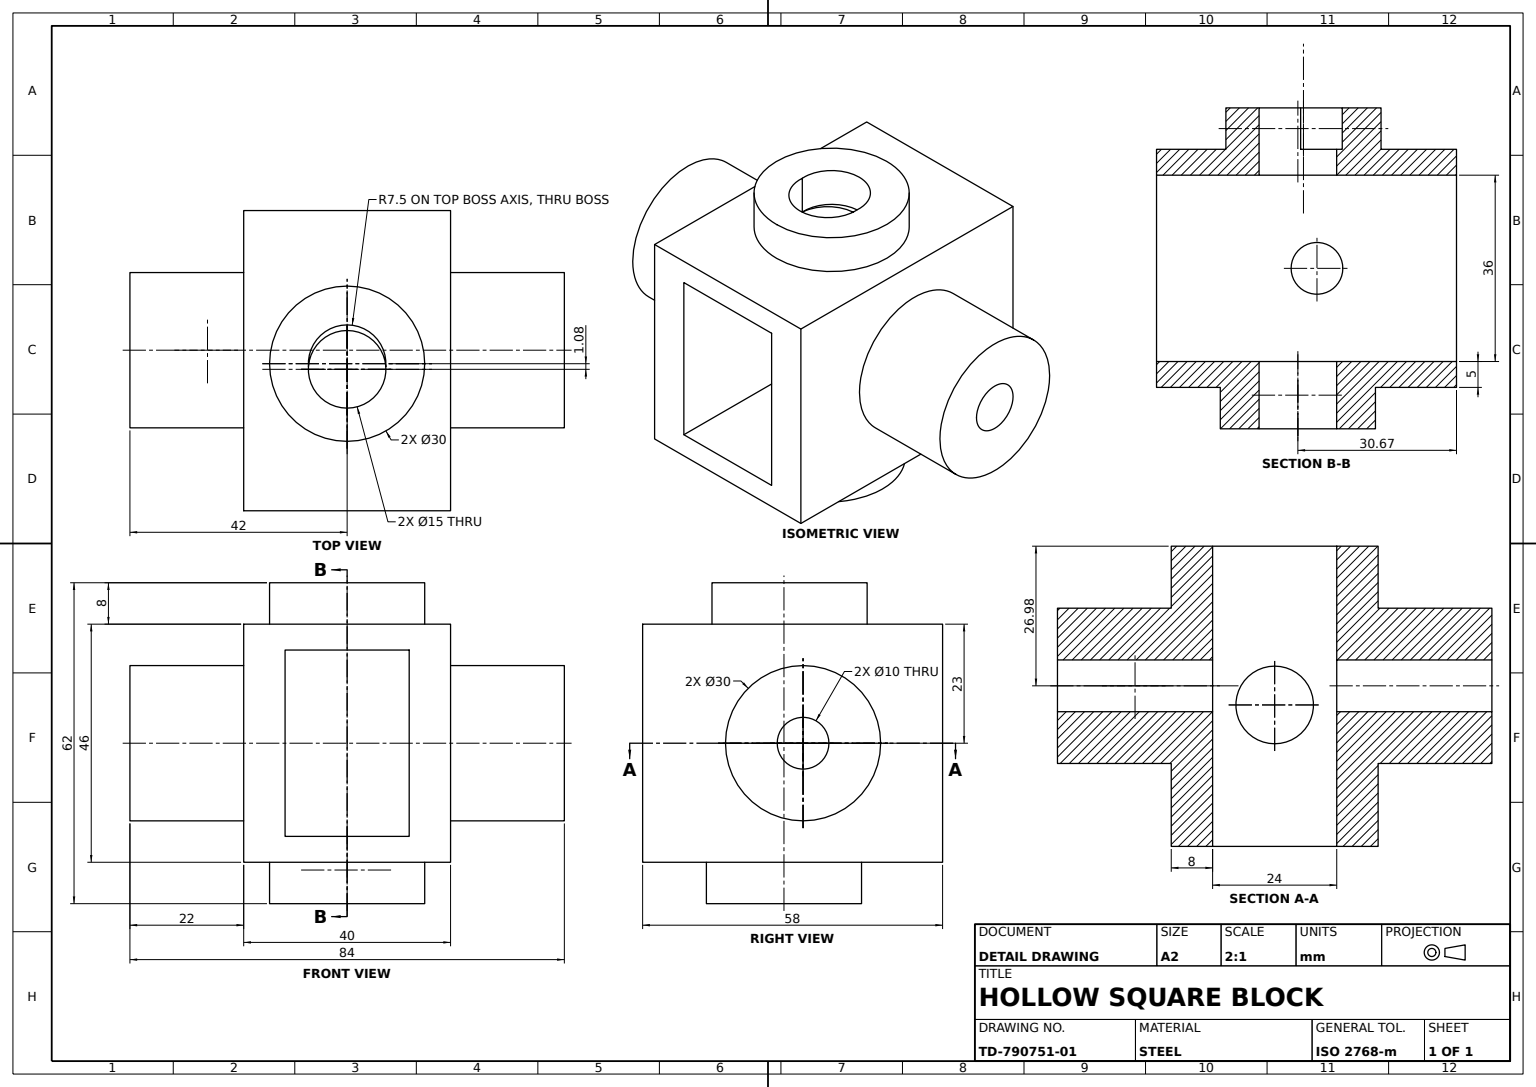
from build123d import *

# Parameters (mm, degrees)
VALVE_BODY_PROFILE_SKETCH_W  = 84
VALVE_BODY_PROFILE_SKETCH_H  = 46
VALVE_BODY_BLOCK_DEPTH       = 23
TOP_PORT_BOSS_SKETCH_R       = 15
TOP_PORT_BOSS_SKETCH_R_2     = 7.5
TOP_PORT_BOSS_30_DEPTH       = 8
BODY_WINDOW_SKETCH_W         = 24
BODY_WINDOW_SKETCH_H         = 36
BODY_WINDOW_CUT_24X36_DEPTH  = 60
SIDE_PORT_SKETCH_R           = 5
SIDE_PORT_THROUGH_BORE_DEPTH = 95
SKETCH4_3_R                  = 15
SKETCH4_3_R_2                = 5
SIDE_PORT_CUT_DEPTH          = 22
REAR_START                   = -22
REAR_PORT_SKETCH_W           = 46
REAR_PORT_SKETCH_H           = 46
REAR_PORT_SKETCH_R           = 15
REAR_PORT_CUT_DEPTH          = 22
FRONT_PORT_BOSS_SKETCH_R     = 15
FRONT_PORT_BOSS_SKETCH_R_2   = 7.5
FRONT_PORT_BOSS_30_DEPTH     = 8
FRONT_START                  = -61
SKETCH6_3_R                  = 7.5
FRONT_PORT_BORE_DEPTH        = 61


with BuildPart() as part:
    # Valve Body Profile Sketch → Valve Body Block (new, symmetric)
    with BuildSketch(Plane(origin=(0, 0, 0), x_dir=(1, 0, 0), z_dir=(0, 1, 0))):
        with Locations((0, 23)):
            Rectangle(VALVE_BODY_PROFILE_SKETCH_W, VALVE_BODY_PROFILE_SKETCH_H)
        Polygon((-20, 51.769982338), (20, 51.769982338), (20, 22.392939221), (20, -6.230017662), (-20, -6.230017662), (-20, 23), align=None)
    extrude(amount=VALVE_BODY_BLOCK_DEPTH, both=True)

    # Top Port Boss Sketch → Top Port Boss _30 (add)
    with BuildSketch(Plane(origin=(0, 23, 0), x_dir=(1, 0, 0), z_dir=(0, 1, 0))):
        with Locations(Location((0, 22.179634707, 0), (0, 0, 270))):
            Circle(TOP_PORT_BOSS_SKETCH_R)
        with Locations(Location((0, 22.179634707, 0), (0, 0, 270))):
            Circle(TOP_PORT_BOSS_SKETCH_R_2, mode=Mode.SUBTRACT)
    extrude(amount=TOP_PORT_BOSS_30_DEPTH)

    # Body Window Sketch → Body Window Cut 24x36 (cut)
    with BuildSketch(Plane.XY.offset(6.230017662)):
        Rectangle(BODY_WINDOW_SKETCH_W, BODY_WINDOW_SKETCH_H)
    extrude(amount=-BODY_WINDOW_CUT_24X36_DEPTH, mode=Mode.SUBTRACT)

    # Side Port Sketch → Side Port Through Bore (cut)
    with BuildSketch(Plane(origin=(42, 0, 0), x_dir=(0, 0, -1), z_dir=(1, 0, 0))):
        with Locations((24.791188033, 0)):
            Circle(SIDE_PORT_SKETCH_R)
    extrude(amount=-SIDE_PORT_THROUGH_BORE_DEPTH, mode=Mode.SUBTRACT)

    # Sketch4_3 → Side Port Cut (cut)
    # profile 1 of 2: a face of its own
    with BuildSketch(Plane(origin=(42, 0, 0), x_dir=(0, 0, -1), z_dir=(1, 0, 0))):
        Polygon((23.784682636, 23), (46, 23), (46, -23), (0, -23), (0, 23), align=None)
        with Locations((24.791188033, 0)):
            Circle(SKETCH4_3_R, mode=Mode.SUBTRACT)
    # profile 2 of 2: a face of its own
    with BuildSketch(Plane(origin=(42, 0, 0), x_dir=(0, 0, -1), z_dir=(1, 0, 0))):
        with Locations((24.791188033, 0)):
            Circle(SKETCH4_3_R_2)
    extrude(amount=-SIDE_PORT_CUT_DEPTH, mode=Mode.SUBTRACT)

    # Rear Port Sketch → Rear Port Cut (cut)
    with BuildSketch(Plane.ZY.offset(42).offset(REAR_START)):
        with Locations((-23, 0)):
            Rectangle(REAR_PORT_SKETCH_W, REAR_PORT_SKETCH_H)
        with Locations(Location((-24.791188033, 0, 0), (0, 0, 180))):
            Circle(REAR_PORT_SKETCH_R, mode=Mode.SUBTRACT)
    extrude(amount=REAR_PORT_CUT_DEPTH, mode=Mode.SUBTRACT)

    # Front Port Boss Sketch → Front Port Boss _30 (add)
    with BuildSketch(Plane.XZ.offset(23)):
        with Locations(Location((0, -21.097330719, 0), (0, 0, 90))):
            Circle(FRONT_PORT_BOSS_SKETCH_R)
        with Locations(Location((0, -21.097330719, 0), (0, 0, 270))):
            Circle(FRONT_PORT_BOSS_SKETCH_R_2, mode=Mode.SUBTRACT)
    extrude(amount=FRONT_PORT_BOSS_30_DEPTH)

    # Sketch6_3 → Front Port Bore (cut)
    with BuildSketch(Plane.XZ.offset(23).offset(FRONT_START)):
        with Locations(Location((0, -21.097330719, 0), (0, 0, 270))):
            Circle(SKETCH6_3_R)
    extrude(amount=FRONT_PORT_BORE_DEPTH, mode=Mode.SUBTRACT)


solid = part.part
